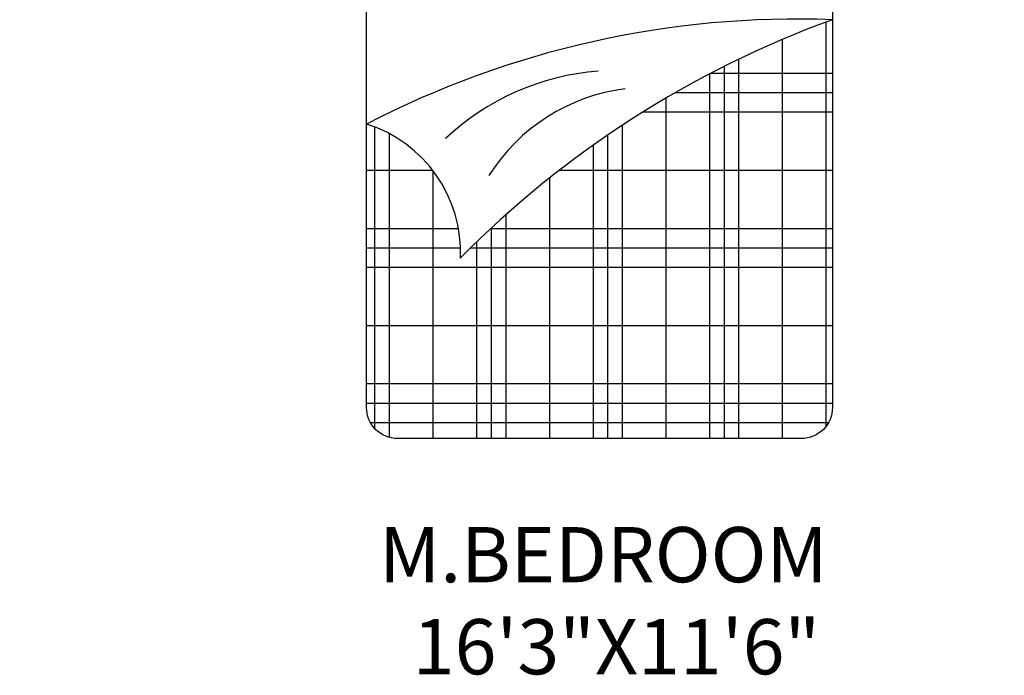
# Model space of a CAD drawing. Units: inches. Extents: x 3064 to 19385, y 846 to 15425.
# Tile 45 of 108: x 5356 to 5481, y 1285 to 1368. Entities that reach past the tile are written whole.
import ezdxf

# ---------------------------------------------------------------- set-up
doc = ezdxf.new("R2010")
doc.units = ezdxf.units.IN
for name, color, linetype, lineweight in [('A-ANNO-DIMS', 2, 'Continuous', 18), ('A-AREA-IDEN', 3, 'Continuous', 18), ('A-FLOR-FIXT', 9, 'Continuous', 18)]:
    doc.layers.add(name, color=color, linetype=linetype, lineweight=lineweight)
doc.layers.add('BLOCK', color=6, linetype='Continuous')
doc.styles.get("Standard").update_dxf_attribs({"font": 'arial.ttf'})
doc.dimstyles.new('ISO-25', dxfattribs={"dimtxt": 9, "dimasz": 2.5, "dimexe": 1.25, "dimexo": 0.625, "dimtad": 1, "dimdec": 1, "dimlunit": 3, "dimtxsty": 'Standard', "dimcen": 2.5, "dimadec": 0, "dimazin": 0, "dimtfac": 1, "dimtdec": 1, "dimtmove": 0, "dimatfit": 3, "dimfxl": 1, "dimarcsym": 0})

# ---------------------------------------------------------------- blocks, each defined once
blk = doc.blocks.new('*X5')
at = {"color": 0}
for p, q in [((276.598, 451.25), (280.51, 451.25)), ((275.455, 450.625), (280.51, 450.625)), ((274.411, 450), (280.51, 450)), ((265.51, 448.125), (267.634, 448.125)), ((271.723, 448.125), (280.51, 448.125)), ((265.51, 446.25), (268.465, 446.25)), ((269.519, 446.25), (280.51, 446.25)), ((265.51, 445.625), (268.531, 445.625)), ((268.866, 445.625), (280.51, 445.625)), ((265.51, 445), (280.51, 445)), ((265.51, 443.125), (280.51, 443.125)), ((265.51, 441.25), (280.51, 441.25)), ((265.51, 440.625), (280.51, 440.625)), ((265.634, 440), (280.386, 440))]:
    blk.add_line(p, q, dxfattribs=at)
blk = doc.blocks.new('*X6')
at = {"color": 0}
for p, q in [((280.312, 439.886), (280.312, 452.896)), ((278.906, 439.482), (278.906, 452.338)), ((277.031, 439.482), (277.031, 451.471)), ((277.5, 439.482), (277.5, 451.702)), ((276.562, 439.482), (276.562, 451.231)), ((275.156, 439.482), (275.156, 450.451)), ((273.75, 439.482), (273.75, 449.576)), ((265.781, 439.797), (265.781, 449.511)), ((266.25, 439.517), (266.25, 449.296)), ((273.281, 439.482), (273.281, 449.261)), ((272.812, 439.482), (272.812, 448.934)), ((267.656, 439.482), (267.656, 448.095)), ((271.406, 439.482), (271.406, 447.876)), ((270, 439.482), (270, 446.689)), ((269.531, 439.482), (269.531, 446.262)), ((269.062, 439.482), (269.062, 445.817))]:
    blk.add_line(p, q, dxfattribs=at)
blk = doc.blocks.new('A$C52E67D0D')
at = {"layer": 'BLOCK'}
blk.add_lwpolyline([(1901, 0), (601, 0, -0.414214), (501, 100), (501, 1700, -0.414214), (601, 1800), (1901, 1800, -0.414214), (2001, 1700), (2001, 100, -0.414214)], format="xyb", close=True, dxfattribs=at)
for centre, radius, start, end in [((1888.6, -1664.5), 3015.3, 87.8642, 117.4001), ((3101, -1685.8), 3227.7, 109.926, 135.3977), ((1308.8, 377.9), 807.6, 94.4436, 133.2788), ((1410.8, 520.2), 610.8, 97.2157, 147.6656), ((371.4, 600.4), 432, 357.3792, 72.5379)]:
    blk.add_arc(centre, radius, start, end, dxfattribs=at)
at = {"layer": 'BLOCK', "xscale": 100, "yscale": 100, "zscale": 100}
for name in ['*X6', '*X5']:
    blk.add_blockref(name, (-26050, -43948.2), dxfattribs=at)
blk = doc.blocks.new('*D443')
at = {"layer": 'A-ANNO-DIMS', "color": 0, "lineweight": -2, "transparency": 16777216}
for p, q in [((5356.02, 1385.47), (5356.02, 1379.45)), ((5392.02, 1385.47), (5392.02, 1379.45)), ((5358.52, 1380.7), (5389.52, 1380.7)), ((5392.02, 1380.7), (5506.9, 1380.7))]:
    blk.add_line(p, q, dxfattribs=at)
at = {"layer": 'A-ANNO-DIMS', "color": 0, "transparency": 16777216}
for points in [[(5358.52, 1381.11), (5358.52, 1380.28), (5356.02, 1380.7)], [(5389.52, 1381.11), (5389.52, 1380.28), (5392.02, 1380.7)]]:
    blk.add_solid(points, dxfattribs=at)
at = {"layer": 'Defpoints', "color": 0, "transparency": 16777216}
for p in [(5356.02, 1386.1), (5392.02, 1386.1), (5392.02, 1380.7)]:
    blk.add_point(p, dxfattribs=at)
at = {"layer": 'A-ANNO-DIMS', "color": 0, "transparency": 16777216, "insert": (5450.71, 1385.92), "char_height": 9, "attachment_point": 5}
blk.add_mtext('W1000-B 3\'-0" TYP.', dxfattribs=at)

msp = doc.modelspace()

# ---------------------------------------------------------------- block references
at = {"layer": 'A-FLOR-FIXT', "xscale": 0.039370099999992, "yscale": 0.039370099999992, "zscale": 0.039370099999992}
msp.add_blockref('A$C52E67D0D', (5380.26, 1315.23), dxfattribs=at)

# ---------------------------------------------------------------- texts
at = {"layer": 'A-AREA-IDEN', "insert": (5401.57, 1304.01), "char_height": 7, "attachment_point": 1}
msp.add_mtext_dynamic_manual_height_columns('M.BEDROOM\\P  16\'3"X11\'6"', width=67.5924, gutter_width=12.5, heights=[0], dxfattribs=at)

# ---------------------------------------------------------------- dimensions: what is measured, and where the dimension line sits
at = {"layer": 'A-ANNO-DIMS'}
dim = msp.add_linear_dim(base=(5392.02, 1380.7), p1=(5356.02, 1386.1), p2=(5392.02, 1386.1), text='W1000-B <> TYP.', dimstyle='ISO-25', override={"dimdec": 1, "dimrnd": 0, "dimzin": 1, "dimlunit": 4, "dimfrac": 2}, dxfattribs=at)
dim.commit()
dim.dimension.update_dxf_attribs({"geometry": '*D443', "text_midpoint": (5450.71, 1385.92)})

doc.saveas('drawing.dxf')
